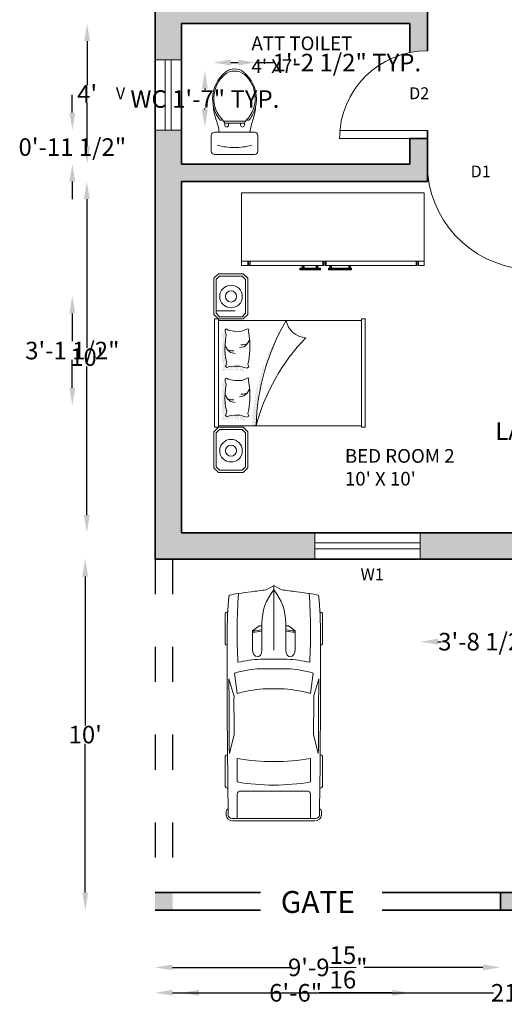
# Model space of a CAD drawing. Units: inches. Extents: x 2178 to 3409, y 1711 to 2279.
# Tile 1 of 8: x 2178 to 2343, y 1711 to 2047. Entities that reach past the tile are written whole.
import ezdxf

# ---------------------------------------------------------------- set-up
doc = ezdxf.new("R2010")
doc.units = ezdxf.units.IN
doc.linetypes.add('ACAD_ISO03W100', pattern=[30, 12, -18])
for name, color, linetype, lineweight in [('A-ANNO-DIMS', 2, 'Continuous', 18), ('A-ANNO-IDEN', 3, 'Continuous', 18), ('A-ANNO-TEXT', 7, 'Continuous', 18), ('A-AREA-IDEN', 7, 'Continuous', 18), ('A-DOOR', 4, 'Continuous', 18), ('A-EQPM-VEHI', 8, 'Continuous', 13), ('A-FURN', 8, 'Continuous', 18), ('A-GLAZ', 4, 'Continuous', 18), ('A-WALL', 7, 'Continuous', 35), ('A-WALL-HIDN', 7, 'ACAD_ISO03W100', 25), ('A-WALL-PATT', 252, 'Continuous', 13), ('WC-Detail_dwgmodels.com', 240, 'Continuous', 13), ('WC-Outline_dwgmodels.com', 250, 'Continuous', 18)]:
    doc.layers.add(name, color=color, linetype=linetype, lineweight=lineweight)
doc.styles.get("Standard").update_dxf_attribs({"font": 'arial.ttf'})
doc.dimstyles.get("Standard").update_dxf_attribs({"dimtxt": 6, "dimasz": 6, "dimexe": 0.18, "dimexo": 0.0625, "dimgap": 0.09, "dimtad": 0, "dimtih": 1, "dimtoh": 1, "dimdec": 4, "dimzin": 0, "dimdsep": 46, "dimlunit": 4, "dimtxsty": 'Standard', "dimcen": 0.09, "dimse1": 1, "dimse2": 1, "dimadec": 0, "dimazin": 0, "dimtfac": 1, "dimtdec": 4, "dimtofl": 0, "dimtmove": 0, "dimatfit": 3, "dimfxl": 1, "dimtolj": 1, "dimtzin": 0, "dimarcsym": 0})
pattern_1 = [(90, (3285.2007, -5256.0159), (-0.408110856, 0.204055428), [0, -0.408110856])]
pattern_2 = [(2e-12, (221.4576, -2145.7372), (1.73228346, -0.78740157), [11.8110236, -1.574803, 3.937008, -0.7874016]), (2e-12, (222.5049, -2146.1309), (-0.7874016, -1.0472441), [2.3622047, -0.2598425, 4.7244094, -0.5905512]), (2e-12, (221.8513, -2146.4065), (4.09448819, -0.52755906), [6.2992126, -1.1023622, 3.1496063, -0.7874016])]

# ---------------------------------------------------------------- blocks, each defined once
blk = doc.blocks.new('*U10')
for p, q in [((536, 950), (536, 936)), ((1182, 988), (568, 988)), ((1214, 950), (1214, 950)), ((2235, 810), (1899, 912)), ((3412, 904), (3030, 807)), ((3440, 942), (3440, 950)), ((3472, 988), (4087, 988)), ((4119, 950), (4119, 934)), ((4736, -851), (4736, 851)), ((4785, -832), (4785, 832)), ((1779, 801), (2195, 746)), ((3516, 746), (3994, 746)), ((4179, 670), (4179, -670)), ((4736, 746), (4242, 746)), ((820, 295), (918, 436)), ((918, 436), (1294, 436)), ((756, 241), (1313, 241)), ((816, 241), (816, 283)), ((1496, -274), (1496, 274)), ((1690, -267), (1690, 267)), ((2102, 216), (2102, -216)), ((4736, -267), (4736, 267)), ((83, 156), (3, 10)), ((0, 0), (1313, 0)), ((3, -10), (83, -156)), ((756, -241), (1313, -241)), ((816, -241), (816, -283)), ((820, -295), (918, -436)), ((918, -436), (1294, -436)), ((2195, -746), (1779, -801)), ((3994, -746), (3516, -746)), ((4242, -746), (4736, -746)), ((536, -950), (536, -936)), ((1182, -988), (568, -988)), ((1214, -950), (1214, -950)), ((2235, -810), (1899, -912)), ((3412, -904), (3030, -807)), ((3440, -942), (3440, -950)), ((3472, -988), (4087, -988)), ((4119, -950), (4119, -934))]:
    blk.add_line(p, q)
for centre, major_axis, ratio, start_param, end_param in [((6757, -699), (0, 7958), 0.842304, 1.367076, 1.39176), ((1046, -12468), (0, 13417), 0.842304, 0.00281, 0.075598), ((568, 950), (0, -37.6), 0.842304, 3.141593, 4.712389), ((1638, -268113), (0, 269063), 0.842304, -0.013397, 0.002797), ((1182, 950), (0, 37.6), 0.842304, -1.570796, 0), ((1638, -268113), (0, -269025), 0.842304, 3.133765, 3.140441), ((2433, -93125), (0, -93935), 0.842304, 3.134049, 3.144098), ((3472, 950), (0, -37.6), 0.842304, 3.141593, 4.712389), ((4087, 950), (0, 37.6), 0.842304, -1.570796, 0), ((4588, 910), (0, 56.4), 0.842304, -0.013017, 1.249894), ((1638, -268131), (0, 269121), 0.842304, -0.013397, -0.013017), ((4673, 851), (0, -75.2), 0.842304, 1.570796, 3.128196), ((4673, 832), (0, -133), 0.842304, 1.570796, 3.128196), ((6583, -699), (0, -7755), 0.842304, 4.528606, 4.561838), ((952, -15087), (0, -15833), 0.842304, 3.096046, 3.200911), ((3414, 137), (0, -2280), 0.842304, 4.449482, 4.652344), ((3436, 137), (0, 2077), 0.842304, 1.245306, 1.50788), ((3800, 71), (0, -2021), 0.842304, 4.372215, 4.640744), ((434, 0), (0, 3734), 0.842304, 4.511394, 4.913384), ((912, 0), (0, 3734), 0.842304, 4.511394, 4.913384), ((4242, 670), (0, 75.2), 0.842304, 0, 1.570796), ((-5194, 1331), (0, -6374), 0.842304, 1.385369, 1.434372), ((331, 432), (0, 696), 0.842304, 4.435146, 4.718221), ((361, 432), (0, 696), 0.842304, 4.435146, 4.718221), ((1290, 339), (161, -9), 0.603834, -1.395552, 1.581315), ((756, -1185), (0, 1427), 0.842304, 0, 0.590319), ((832, 283), (0, 18.8), 0.842304, 0.879714, 1.570796), ((16, 0), (0, -18.8), 0.842304, 4.131459, 5.293319), ((-5194, -1331), (0, 6374), 0.842304, -1.434372, -1.385369), ((756, 1185), (0, 1427), 0.842304, 2.551274, 3.141593), ((832, -283), (0, -18.8), 0.842304, 4.712389, 5.403472), ((331, -432), (0, -696), 0.842304, 1.564964, 1.848039), ((361, -432), (0, -696), 0.842304, 1.564964, 1.848039), ((3414, -137), (0, -2280), 0.842304, -1.510751, -1.307889), ((3436, -137), (0, -2077), 0.842304, -1.50788, -1.245306), ((3800, -71), (0, -2021), 0.842304, -1.499151, -1.230623), ((6583, 699), (0, 7755), 0.842304, 1.721348, 1.754579), ((6757, 699), (0, 7958), 0.842304, 1.749832, 1.774517), ((952, 15087), (0, -15833), 0.842304, -0.059319, 0.045547), ((4242, -670), (0, -75.2), 0.842304, 4.712389, 6.283185), ((1046, 12468), (0, -13417), 0.842304, -0.075598, -0.00281), ((568, -950), (0, 37.6), 0.842304, 1.570796, 3.141593), ((1638, 268113), (0, 269063), 0.842304, 3.138796, 3.15499), ((1182, -950), (0, -37.6), 0.842304, 0, 1.570796), ((1638, 268113), (0, -269025), 0.842304, 0.001152, 0.007828), ((2433, 93125), (0, -93935), 0.842304, -0.002505, 0.007544), ((3472, -950), (0, -37.6), 0.842304, -1.570796, 0), ((4087, -950), (0, 37.6), 0.842304, 3.141593, 4.712389), ((4588, -910), (0, -56.4), 0.842304, -1.249894, 0.013017), ((1638, 268131), (0, 269121), 0.842304, 3.15461, 3.15499), ((4673, -851), (0, 75.2), 0.842304, 3.15499, 4.712389), ((4673, -832), (0, -133), 0.842304, 0.013397, 1.570796)]:
    blk.add_ellipse(centre, major_axis=major_axis, ratio=ratio, start_param=start_param, end_param=end_param)
at = {"extrusion": (0, 0, -1)}
blk.add_ellipse((1290, -339), major_axis=(161, 9), ratio=0.603834, start_param=-1.395552, end_param=1.581315, dxfattribs=at)
blk = doc.blocks.new('*D13')
at = {"layer": 'A-ANNO-DIMS', "color": 0, "lineweight": -2, "transparency": 16777216}
for p, q in [((2200.86, 2040.04), (2200.86, 2025.13)), ((2200.86, 2004.04), (2200.86, 2018.95))]:
    blk.add_line(p, q, dxfattribs=at)
at = {"layer": 'A-ANNO-DIMS', "color": 0, "transparency": 16777216}
for points in [[(2199.86, 2040.04), (2201.86, 2040.04), (2200.86, 2046.04)], [(2199.86, 2004.04), (2201.86, 2004.04), (2200.86, 1998.04)]]:
    blk.add_solid(points, dxfattribs=at)
at = {"layer": 'Defpoints', "color": 0, "transparency": 16777216}
for p in [(2278.29, 2046.04), (2200.86, 1998.04), (2281.09, 1998.04)]:
    blk.add_point(p, dxfattribs=at)
at = {"layer": 'A-ANNO-DIMS', "color": 0, "transparency": 16777216, "insert": (2200.86, 2022.04), "char_height": 6, "width": 5.7626, "attachment_point": 5}
blk.add_mtext("\\A1;4'", dxfattribs=at)
blk = doc.blocks.new('*D14')
at = {"layer": 'A-ANNO-DIMS', "color": 0, "lineweight": -2, "transparency": 16777216}
for p, q in [((2200.76, 1986.04), (2200.76, 1935.2)), ((2200.76, 1878.04), (2200.76, 1928.89))]:
    blk.add_line(p, q, dxfattribs=at)
at = {"layer": 'A-ANNO-DIMS', "color": 0, "transparency": 16777216}
for points in [[(2199.76, 1986.04), (2201.76, 1986.04), (2200.76, 1992.04)], [(2199.76, 1878.04), (2201.76, 1878.04), (2200.76, 1872.04)]]:
    blk.add_solid(points, dxfattribs=at)
at = {"layer": 'Defpoints', "color": 0, "transparency": 16777216}
for p in [(2275.06, 1992.04), (2200.76, 1872.04), (2275.06, 1872.04)]:
    blk.add_point(p, dxfattribs=at)
at = {"layer": 'A-ANNO-DIMS', "color": 0, "transparency": 16777216, "insert": (2200.76, 1932.04), "char_height": 6, "attachment_point": 5}
blk.add_mtext("\\A1;10'", dxfattribs=at)
blk = doc.blocks.new('*D15')
at = {"layer": 'A-ANNO-DIMS', "color": 0, "lineweight": -2, "transparency": 16777216}
for p, q in [((2200.22, 1857.04), (2200.22, 1806.2)), ((2200.22, 1749.04), (2200.22, 1799.89))]:
    blk.add_line(p, q, dxfattribs=at)
at = {"layer": 'A-ANNO-DIMS', "color": 0, "transparency": 16777216}
for points in [[(2199.22, 1857.04), (2201.22, 1857.04), (2200.22, 1863.04)], [(2199.22, 1749.04), (2201.22, 1749.04), (2200.22, 1743.04)]]:
    blk.add_solid(points, dxfattribs=at)
at = {"layer": 'Defpoints', "color": 0, "transparency": 16777216}
for p in [(2238.48, 1863.04), (2200.22, 1743.04), (2238.48, 1743.04)]:
    blk.add_point(p, dxfattribs=at)
at = {"layer": 'A-ANNO-DIMS', "color": 0, "transparency": 16777216, "insert": (2200.22, 1803.04), "char_height": 6, "attachment_point": 5}
blk.add_mtext("\\A1;10'", dxfattribs=at)
blk = doc.blocks.new('*D16')
at = {"layer": 'A-ANNO-DIMS', "color": 0, "lineweight": -2, "transparency": 16777216}
for p, q in [((2230.06, 1723.48), (2270.74, 1723.48)), ((2336.02, 1723.48), (2295.35, 1723.48))]:
    blk.add_line(p, q, dxfattribs=at)
at = {"layer": 'A-ANNO-DIMS', "color": 0, "transparency": 16777216}
for points in [[(2230.06, 1724.48), (2230.06, 1722.48), (2224.06, 1723.48)], [(2336.02, 1724.48), (2336.02, 1722.48), (2342.02, 1723.48)]]:
    blk.add_solid(points, dxfattribs=at)
at = {"layer": 'Defpoints', "color": 0, "transparency": 16777216}
for p in [(2224.06, 1743.04), (2342.02, 1743.04), (2342.02, 1723.48)]:
    blk.add_point(p, dxfattribs=at)
at = {"layer": 'A-ANNO-DIMS', "color": 0, "transparency": 16777216, "insert": (2283.04, 1723.48), "char_height": 6, "attachment_point": 5}
blk.add_mtext('\\A1;9\'-9{\\H1x;\\S15/16;}"', dxfattribs=at)
blk = doc.blocks.new('BED-WITH-NIGHTSTANDS')
h = blk.add_hatch()
h.set_pattern_fill('DOTS', color=256, scale=0.257078, angle=90, style=0)
h.set_pattern_definition(pattern_1)
h.paths.add_polyline_path([(12.63, 18.62), (14.4, 18.62, -0.124273), (24.68, 54.62, 0.122563)])
h = blk.add_hatch()
h.set_pattern_fill('DOTS', color=256, scale=0.257078, angle=90, style=0)
h.set_pattern_definition(pattern_1)
h.paths.add_polyline_path([(3.05, 33.63), (2.57, 33.32), (2.57, 32.61), (2.97, 31.58), (2.65, 29.84), (2.42, 26.52), (2.65, 23.75), (3.13, 22.32), (2.65, 20.82), (3.28, 20.43), (4, 20.74), (5.81, 20.9), (7.55, 20.9), (9.13, 20.51), (10, 20.27), (10.71, 20.66), (10.32, 21.53), (10.39, 21.79), (8.83, 22.19), (7.1, 22.19), (5.28, 22.03), (4.57, 21.71), (3.93, 22.11), (4.41, 23.61), (3.93, 25.03), (3.7, 27.8), (3.93, 31.12), (4.25, 32.86), (4.14, 33.14), (3.6, 33.24)])
h.paths.add_polyline_path([(3.05, 50.43), (2.57, 50.11), (2.57, 49.4), (2.97, 48.37), (2.65, 46.63), (2.42, 43.31), (2.65, 40.54), (3.13, 39.12), (2.65, 37.62), (3.28, 37.22), (4, 37.54), (5.81, 37.7), (7.55, 37.7), (9.13, 37.3), (10, 37.06), (10.71, 37.46), (10.32, 38.33), (10.39, 38.59), (8.83, 38.98), (7.1, 38.98), (5.28, 38.82), (4.57, 38.51), (3.93, 38.9), (4.41, 40.4), (3.93, 41.83), (3.7, 44.59), (3.93, 47.92), (4.25, 49.66), (4.14, 49.93), (3.6, 50.03)])
for p, q in [((0.8, 57.9), (7.23, 57.9)), ((0.26, 55.13), (0.26, 18.11)), ((0.26, 55.13), (1.54, 55.13)), ((1.54, 55.13), (1.54, 18.11)), ((1.54, 54.62), (50.39, 54.62)), ((50.39, 55.13), (50.39, 18.11)), ((50.39, 55.13), (51.67, 55.13)), ((51.67, 55.13), (51.67, 18.11)), ((1.54, 18.11), (0.26, 18.11)), ((50.39, 18.62), (1.54, 18.62)), ((51.67, 18.11), (50.39, 18.11))]:
    blk.add_line(p, q)
for points in [[(11.57, 56.67), (11.57, 69.01), (10.03, 70.55), (1.54, 70.55), (0, 69.01), (0, 56.67), (1.54, 55.13), (10.03, 55.13)], [(10.8, 57.06), (10.8, 68.63), (9.64, 69.78), (1.93, 69.78), (0.77, 68.63), (0.77, 57.06), (1.93, 55.9), (9.64, 55.9)], [(11.57, 4.23), (11.57, 16.57), (10.03, 18.11), (1.54, 18.11), (0, 16.57), (0, 4.23), (1.54, 2.69), (10.03, 2.69)], [(10.8, 4.61), (10.8, 16.18), (9.64, 17.34), (1.93, 17.34), (0.77, 16.18), (0.77, 4.61), (1.93, 3.46), (9.64, 3.46)]]:
    blk.add_lwpolyline(points, close=True)
for points in [[(4.41, 40.4), (3.93, 38.9), (4.57, 38.51), (5.28, 38.82), (7.1, 38.98), (8.83, 38.98), (10.41, 38.58), (11.28, 38.35), (11.99, 38.74), (11.6, 39.61), (11.99, 40.96), (12.23, 44.2), (12.23, 47.52), (11.84, 51), (11.99, 51.63), (11.6, 51.79), (10.97, 51.47), (9.54, 50.92), (7.17, 50.84), (5.75, 51.16), (4.88, 51.32), (4.33, 51.71), (3.86, 51.4), (3.86, 50.68), (4.25, 49.66), (3.93, 47.92), (3.7, 44.59), (3.93, 41.83), (4.41, 40.4)], [(12.15, 47.92), (11.36, 46.57), (10.33, 45.62), (8.75, 45.31)], [(3.86, 45.94), (4.65, 44.59), (5.67, 43.65), (7.25, 43.33)], [(4.72, 44.59), (5.99, 44.28), (6.78, 44.28)], [(11.28, 46.57), (10.02, 46.26), (9.23, 46.26)], [(4.41, 23.61), (3.93, 22.11), (4.57, 21.71), (5.28, 22.03), (7.1, 22.19), (8.83, 22.19), (10.41, 21.79), (11.28, 21.55), (11.99, 21.95), (11.6, 22.82), (11.99, 24.16), (12.23, 27.4), (12.23, 30.73), (11.84, 34.21), (11.99, 34.84), (11.6, 35), (10.97, 34.68), (9.54, 34.13), (7.17, 34.05), (5.75, 34.36), (4.88, 34.52), (4.33, 34.92), (3.86, 34.6), (3.86, 33.89), (4.25, 32.86), (3.93, 31.12), (3.7, 27.8), (3.93, 25.03), (4.41, 23.61)], [(12.15, 31.12), (11.36, 29.78), (10.33, 28.83), (8.75, 28.51)], [(3.86, 29.14), (4.65, 27.8), (5.67, 26.85), (7.25, 26.53)], [(4.72, 27.8), (5.99, 27.48), (6.78, 27.48)], [(11.28, 29.78), (10.02, 29.46), (9.23, 29.46)]]:
    blk.add_lwpolyline(points)
for centre, radius in [((5.86, 62.82), 3.86), ((5.86, 62.82), 1.91), ((5.86, 10.09), 3.86), ((5.86, 10.09), 1.91)]:
    blk.add_circle(centre, radius)
for centre, radius, start, end in [((90.82, 16.25), 76.46, 149.8866, 178.2226), ((31.77, 55.91), 7.21, 190.3543, 266.7862), ((82.59, 0), 70.69, 136.4367, 164.7234)]:
    blk.add_arc(centre, radius, start, end)
blk = doc.blocks.new('BEDROOM-WARDROBE')
h = blk.add_hatch()
h.set_pattern_fill('AR-RROOF', color=256, scale=0.787402, angle=360, style=0)
h.set_pattern_definition(pattern_2)
h.paths.add_polyline_path([(19.88, 0.59), (19.88, 0), (26.97, 0), (26.97, 0.59)])
h.paths.add_polyline_path([(26.07, 1.57), (25.48, 1.57), (25.48, 0.59), (26.07, 0.59)])
h.paths.add_polyline_path([(21.37, 1.57), (20.78, 1.57), (20.78, 0.59), (21.37, 0.59)])
h = blk.add_hatch()
h.set_pattern_fill('AR-RROOF', color=256, scale=0.787402, angle=360, style=0)
h.set_pattern_definition(pattern_2)
h.paths.add_polyline_path([(29.73, 0.59), (29.73, 0), (37.6, 0), (37.6, 0.59)])
h.paths.add_polyline_path([(37.21, 1.57), (36.61, 1.57), (36.61, 0.59), (37.21, 0.59)])
h.paths.add_polyline_path([(30.71, 0.59), (30.71, 1.57), (30.12, 1.57), (30.12, 0.59)])
for p, q in [((0, 26.38), (62.4, 26.38)), ((0, 26.38), (0, 1.57)), ((62.4, 26.38), (62.4, 1.74)), ((62.4, 2.95), (0, 2.95)), ((0, 1.57), (2.17, 1.57)), ((2.17, 1.57), (2.17, 2.95)), ((2.56, 1.54), (2.56, 2.95)), ((2.95, 1.54), (2.56, 1.54)), ((2.95, 1.57), (2.95, 2.95)), ((27.76, 1.57), (2.95, 1.57)), ((2.95, 1.57), (2.95, 1.54)), ((19.88, 0.59), (26.97, 0.59)), ((19.88, 0), (19.88, 0.59)), ((26.97, 0), (19.88, 0)), ((20.78, 0.59), (20.78, 1.57)), ((21.37, 0.59), (21.37, 1.57)), ((25.48, 0.59), (25.48, 1.57)), ((26.07, 0.59), (26.07, 1.57)), ((26.97, 0.59), (26.97, 0)), ((27.76, 2.95), (27.76, 1.57)), ((27.76, 1.54), (27.76, 1.57)), ((28.15, 1.54), (27.76, 1.54)), ((28.15, 2.95), (28.15, 1.54)), ((28.54, 2.95), (28.54, 1.54)), ((28.54, 1.54), (28.94, 1.54)), ((28.94, 2.95), (28.94, 1.57)), ((28.94, 1.57), (59.65, 1.57)), ((28.94, 1.54), (28.94, 1.57)), ((29.73, 0.59), (37.6, 0.59)), ((29.73, 0), (29.73, 0.59)), ((37.6, 0), (29.73, 0)), ((30.12, 0.59), (30.12, 1.57)), ((30.71, 0.59), (30.71, 1.57)), ((36.61, 0.59), (36.61, 1.57)), ((37.21, 0.59), (37.21, 1.57)), ((37.6, 0.59), (37.6, 0)), ((59.65, 2.95), (59.65, 1.57)), ((59.65, 1.57), (59.65, 1.54)), ((59.65, 1.54), (60.04, 1.54)), ((60.04, 1.54), (60.04, 2.95)), ((60.43, 2.95), (60.43, 1.57))]:
    blk.add_line(p, q)
for centre, radius, start, end in [((61.42, 6.59), 5.11, 258.8892, 279.227), ((62.2, 1.74), 0.197, 279.227, 0)]:
    blk.add_arc(centre, radius, start, end)
blk = doc.blocks.new('WC-SEAT-ASSEMBLY')
for p, q in [((3.53, 1.38), (3.89, 0.72)), ((5.18, 0.72), (3.89, 0.72)), ((3.89, 0.72), (3.89, 0)), ((7.25, 0.72), (5.18, 0.72)), ((5.18, 0), (5.18, 0.72)), ((7.25, 0.72), (9.32, 0.72)), ((9.32, 0.72), (10.61, 0.72)), ((9.32, 0), (9.32, 0.72)), ((10.97, 1.38), (10.61, 0.72)), ((10.61, 0.72), (10.61, 0))]:
    blk.add_line(p, q)
for points in [[(3.26, 1.65, -0.434217), (3.89, 17.29, -0.182634), (7.25, 18.51, -2.693815)], [(11.24, 1.65, 0.434217), (10.61, 17.29, 0.182634), (7.25, 18.51, 2.693815)], [(0.16, 6.03, -0.015301), (0, 6.73, -0.16845)], [(2.36, 1.65, -0.105447), (0.16, 6.03, -0.16845)], [(12.14, 1.65, 0.094048), (14.19, 5.52, 0.16845)], [(14.19, 5.52, 0.026594), (14.5, 6.73, 0.16845)], [(3.26, 1.65), (2.36, 1.65, -0.416606)], [(3.53, 1.38, -0.008985), (3.26, 1.65, -0.182634)], [(7.25, 1.38), (3.53, 1.38, -0.444938)], [(7.25, 1.38), (10.97, 1.38, 0.008985)], [(10.97, 1.38, 0.008985), (11.24, 1.65, 0.182634)], [(11.24, 1.65), (12.14, 1.65, 0.416606)]]:
    blk.add_lwpolyline(points, format="xyb")
for centre in [(4.54, 0), (9.96, 0)]:
    blk.add_arc(centre, 0.645, 180, 0)
blk = doc.blocks.new('WINDOW-36')
for p, q in [((36, 9), (0, 9)), ((0, 9), (0, 0)), ((36, 0), (36, 9)), ((0, 5.5), (36, 5.5)), ((0, 3.5), (36, 3.5)), ((0, 0), (36, 0))]:
    blk.add_line(p, q)
blk = doc.blocks.new('VENT-24')
for p, q in [((9, 24), (0, 24)), ((0, 24), (0, 0)), ((3.5, 0), (3.5, 24)), ((5.5, 0), (5.5, 24)), ((9, 0), (9, 24)), ((0, 0), (9, 0))]:
    blk.add_line(p, q)
blk = doc.blocks.new('DOOR-30')
for p, q in [((-30, 2.75), (0, 2.75)), ((-30, 0), (0, 0)), ((0, 2.75), (0, 0))]:
    blk.add_line(p, q)
blk.add_arc((0, 0), 30, 90, 180)
blk = doc.blocks.new('DOOR-36')
for p, q in [((0, 0), (0, 36)), ((3, 0), (3, 35.87)), ((3, 0), (0, 0))]:
    blk.add_line(p, q)
blk.add_arc((0, 0), 36, 0, 85.2198)
blk = doc.blocks.new('*D45')
at = {"layer": 'A-ANNO-DIMS', "color": 0, "lineweight": -2, "transparency": 16777216}
for p, q in [((2377.15, 1916.05), (2377.15, 1922.05)), ((2377.15, 1897.4), (2377.15, 1891.4))]:
    blk.add_line(p, q, dxfattribs=at)
at = {"layer": 'A-ANNO-DIMS', "color": 0, "transparency": 16777216}
for points in [[(2376.15, 1916.05), (2378.15, 1916.05), (2377.15, 1910.05)], [(2376.15, 1897.4), (2378.15, 1897.4), (2377.15, 1903.4)]]:
    blk.add_solid(points, dxfattribs=at)
at = {"layer": 'Defpoints', "color": 0, "transparency": 16777216}
for p in [(2376.15, 1910.05), (2377.15, 1910.05), (2376.15, 1903.4)]:
    blk.add_point(p, dxfattribs=at)
at = {"layer": 'A-ANNO-DIMS', "color": 0, "transparency": 16777216, "insert": (2377.15, 1906.72), "char_height": 6, "attachment_point": 5}
blk.add_mtext('\\A1;LAMP 0\'-6 1/2" TYP.', dxfattribs=at)
blk = doc.blocks.new('*D51')
at = {"layer": 'A-ANNO-DIMS', "color": 0, "lineweight": -2, "transparency": 16777216}
for p, q in [((2241.08, 2023.86), (2241.08, 2023.46)), ((2241.08, 2016.69), (2241.08, 2017.08))]:
    blk.add_line(p, q, dxfattribs=at)
at = {"layer": 'A-ANNO-DIMS', "color": 0, "transparency": 16777216}
for points in [[(2240.08, 2023.86), (2242.08, 2023.86), (2241.08, 2029.86)], [(2240.08, 2016.69), (2242.08, 2016.69), (2241.08, 2010.69)]]:
    blk.add_solid(points, dxfattribs=at)
at = {"layer": 'Defpoints', "color": 0, "transparency": 16777216}
for p in [(2241.08, 2029.86), (2243.96, 2029.86), (2243.96, 2010.69)]:
    blk.add_point(p, dxfattribs=at)
at = {"layer": 'A-ANNO-DIMS', "color": 0, "transparency": 16777216, "insert": (2241.08, 2020.27), "char_height": 6, "attachment_point": 5}
blk.add_mtext('\\A1;WC 1\'-7" TYP.', dxfattribs=at)
blk = doc.blocks.new('*D52')
at = {"layer": 'A-ANNO-DIMS', "color": 0, "lineweight": -2, "transparency": 16777216}
for p, q in [((2249.96, 2032.73), (2252.46, 2032.73)), ((2258.46, 2032.73), (2264.46, 2032.73))]:
    blk.add_line(p, q, dxfattribs=at)
at = {"layer": 'A-ANNO-DIMS', "color": 0, "transparency": 16777216}
for points in [[(2249.96, 2033.73), (2249.96, 2031.73), (2243.96, 2032.73)], [(2252.46, 2033.73), (2252.46, 2031.73), (2258.46, 2032.73)]]:
    blk.add_solid(points, dxfattribs=at)
at = {"layer": 'Defpoints', "color": 0, "transparency": 16777216}
for p in [(2258.46, 2032.73), (2243.96, 2029.86), (2258.46, 2029.86)]:
    blk.add_point(p, dxfattribs=at)
at = {"layer": 'A-ANNO-DIMS', "color": 0, "transparency": 16777216, "insert": (2289.54, 2032.73), "char_height": 6, "attachment_point": 5}
blk.add_mtext('\\A1;1\'-2 1/2" TYP.', dxfattribs=at)
blk = doc.blocks.new('*D53')
at = {"layer": 'A-ANNO-DIMS', "color": 0, "lineweight": -2, "transparency": 16777216}
for p, q in [((2293.06, 2057.04), (2311.06, 2057.04)), ((2317.06, 2057.04), (2323.06, 2057.04))]:
    blk.add_line(p, q, dxfattribs=at)
at = {"layer": 'A-ANNO-DIMS', "color": 0, "transparency": 16777216}
for points in [[(2293.06, 2058.04), (2293.06, 2056.04), (2287.06, 2057.04)], [(2311.06, 2058.04), (2311.06, 2056.04), (2317.06, 2057.04)]]:
    blk.add_solid(points, dxfattribs=at)
at = {"layer": 'Defpoints', "color": 0, "transparency": 16777216}
for p in [(2287.06, 2061.54), (2317.06, 2061.54), (2317.06, 2057.04)]:
    blk.add_point(p, dxfattribs=at)
at = {"layer": 'A-ANNO-DIMS', "color": 0, "transparency": 16777216, "insert": (2347.81, 2057.04), "char_height": 6, "attachment_point": 5}
blk.add_mtext('\\A1;D2 2\'-6" TYP.', dxfattribs=at)
blk = doc.blocks.new('*D61')
at = {"layer": 'A-ANNO-DIMS', "color": 0, "lineweight": -2, "transparency": 16777216}
for p, q in [((2239.06, 1714.79), (2263.98, 1714.79)), ((2305.06, 1714.79), (2280.15, 1714.79))]:
    blk.add_line(p, q, dxfattribs=at)
at = {"layer": 'A-ANNO-DIMS', "color": 0, "transparency": 16777216}
for points in [[(2239.06, 1715.79), (2239.06, 1713.79), (2233.06, 1714.79)], [(2305.06, 1715.79), (2305.06, 1713.79), (2311.06, 1714.79)]]:
    blk.add_solid(points, dxfattribs=at)
at = {"layer": 'Defpoints', "color": 0, "transparency": 16777216}
for p in [(2233.06, 1998.04), (2311.06, 1998.04), (2311.06, 1714.79)]:
    blk.add_point(p, dxfattribs=at)
at = {"layer": 'A-ANNO-DIMS', "color": 0, "transparency": 16777216, "insert": (2272.06, 1714.79), "char_height": 6, "attachment_point": 5}
blk.add_mtext('\\A1;6\'-6"', dxfattribs=at)
blk = doc.blocks.new('*D63')
at = {"layer": 'A-ANNO-DIMS', "color": 0, "lineweight": -2, "transparency": 16777216}
for p, q in [((2195.814847, 2015.642505), (2195.814847, 2021.642505)), ((2195.814847, 1992.042563), (2195.814847, 1986.042563))]:
    blk.add_line(p, q, dxfattribs=at)
at = {"layer": 'A-ANNO-DIMS', "color": 0, "transparency": 16777216}
for points in [[(2194.814847, 2015.642505), (2196.814847, 2015.642505), (2195.814847, 2009.642505)], [(2194.814847, 1992.042563), (2196.814847, 1992.042563), (2195.814847, 1998.042563)]]:
    blk.add_solid(points, dxfattribs=at)
at = {"layer": 'Defpoints', "color": 0, "transparency": 16777216}
for p in [(2195.814847, 2009.642505), (2233.064847, 2009.642505), (2233.064847, 1998.042563)]:
    blk.add_point(p, dxfattribs=at)
at = {"layer": 'A-ANNO-DIMS', "color": 0, "transparency": 16777216, "insert": (2195.814847, 2003.842534), "char_height": 6, "attachment_point": 5}
blk.add_mtext('\\A1;0\'-11 1/2"', dxfattribs=at)
blk = doc.blocks.new('*D68')
at = {"layer": 'A-ANNO-DIMS', "color": 0, "lineweight": -2, "transparency": 16777216}
for p, q in [((2320.65, 1834.79), (2321.8, 1834.79)), ((2353.06, 1834.79), (2351.91, 1834.79))]:
    blk.add_line(p, q, dxfattribs=at)
at = {"layer": 'A-ANNO-DIMS', "color": 0, "transparency": 16777216}
for points in [[(2320.65, 1835.79), (2320.65, 1833.79), (2314.65, 1834.79)], [(2353.06, 1835.79), (2353.06, 1833.79), (2359.06, 1834.79)]]:
    blk.add_solid(points, dxfattribs=at)
at = {"layer": 'Defpoints', "color": 0, "transparency": 16777216}
for p in [(2314.65, 1863.04), (2359.06, 1863.04), (2314.65, 1834.79)]:
    blk.add_point(p, dxfattribs=at)
at = {"layer": 'A-ANNO-DIMS', "color": 0, "transparency": 16777216, "insert": (2336.86, 1834.79), "char_height": 6, "attachment_point": 5}
blk.add_mtext('\\A1;3\'-8 1/2"', dxfattribs=at)
blk = doc.blocks.new('*D72')
at = {"layer": 'A-ANNO-DIMS', "color": 0, "lineweight": -2, "transparency": 16777216}
for p, q in [((2195.81, 1946.99), (2195.81, 1937.48)), ((2195.81, 1921.59), (2195.81, 1931.1))]:
    blk.add_line(p, q, dxfattribs=at)
at = {"layer": 'A-ANNO-DIMS', "color": 0, "transparency": 16777216}
for points in [[(2194.81, 1946.99), (2196.81, 1946.99), (2195.81, 1952.99)], [(2194.81, 1921.59), (2196.81, 1921.59), (2195.81, 1915.59)]]:
    blk.add_solid(points, dxfattribs=at)
at = {"layer": 'Defpoints', "color": 0, "transparency": 16777216}
for p in [(2195.81, 1952.99), (2366.59, 1952.99), (2366.59, 1915.59)]:
    blk.add_point(p, dxfattribs=at)
at = {"layer": 'A-ANNO-DIMS', "color": 0, "transparency": 16777216, "insert": (2195.81, 1934.29), "char_height": 6, "attachment_point": 5}
blk.add_mtext('\\A1;3\'-1 1/2"', dxfattribs=at)
blk = doc.blocks.new('*D74')
at = {"layer": 'A-ANNO-DIMS', "color": 0, "lineweight": -2, "transparency": 16777216}
for p, q in [((2230.06, 1714.79), (2339.62, 1714.79)), ((2470.06, 1714.79), (2360.51, 1714.79))]:
    blk.add_line(p, q, dxfattribs=at)
at = {"layer": 'A-ANNO-DIMS', "color": 0, "transparency": 16777216}
for points in [[(2230.06, 1715.79), (2230.06, 1713.79), (2224.06, 1714.79)], [(2470.06, 1715.79), (2470.06, 1713.79), (2476.06, 1714.79)]]:
    blk.add_solid(points, dxfattribs=at)
at = {"layer": 'Defpoints', "color": 0, "transparency": 16777216}
for p in [(2224.06, 1743.04), (2476.06, 1743.04), (2476.06, 1714.79)]:
    blk.add_point(p, dxfattribs=at)
at = {"layer": 'A-ANNO-DIMS', "color": 0, "transparency": 16777216, "insert": (2350.06, 1714.79), "char_height": 6, "attachment_point": 5}
blk.add_mtext('\\A1;21\'-0"', dxfattribs=at)

msp = doc.modelspace()

# ---------------------------------------------------------------- hatches: boundary and pattern name
at = {"layer": 'A-WALL-PATT'}
h = msp.add_hatch(color=256, dxfattribs=at)
h.dxf.hatch_style = 1
h.paths.add_polyline_path([(2233.06485, 1992.04256), (2317.06485, 1992.04256), (2317.06485, 1998.04256), (2317.06485, 2006.75072), (2311.06485, 2006.75072), (2311.06485, 1998.04256), (2233.06485, 1998.04256), (2233.06485, 2009.64251), (2224.06485, 2009.64251), (2224.06485, 1863.04256), (2233.06485, 1863.04256), (2278.65041, 1863.04256), (2278.65041, 1872.04256), (2233.06485, 1872.04256)])
h.paths.add_polyline_path([(2359.06485, 1992.04256), (2359.06485, 1998.04256), (2353.06485, 1998.04256), (2353.06485, 1962.04256), (2353.06485, 1872.04256), (2314.65041, 1872.04256), (2314.65041, 1863.04256), (2359.06485, 1863.04256), (2359.06485, 1872.04256)])
h.paths.add_polyline_path([(2401.06485, 1890.04256), (2371.06485, 1890.04256), (2359.06485, 1890.04256), (2359.06485, 1884.04256), (2371.06485, 1884.04256), (2377.06485, 1884.04256), (2401.06485, 1884.04256)])
h.paths.add_polyline_path([(2353.06485, 1802.77269), (2359.06485, 1802.77269), (2359.06485, 1808.77269), (2356.83755, 1808.77269), (2353.06485, 1808.77269), (2347.91295, 1808.77269), (2347.91295, 1802.77269), (2347.91295, 1749.04256), (2342.02347, 1749.04256), (2342.02347, 1743.04256), (2353.06485, 1743.04256)])
h.paths.add_polyline_path([(2476.06485, 2247.04256), (2442.91353, 2247.04256), (2442.91353, 2238.04256), (2467.06485, 2238.04256), (2467.06485, 2041.93675), (2476.06485, 2041.93675)])
h.paths.add_polyline_path([(2467.06485, 2106.04256), (2406.56133, 2106.04256, -0.04188649), (2407.06485, 2100.04256), (2467.06485, 2100.04256)])
h.paths.add_polyline_path([(2406.91353, 2247.04256), (2321.22384, 2247.04256), (2321.22384, 2238.04256), (2365.06485, 2238.04256), (2365.06485, 2106.04256), (2365.06485, 2100.04256), (2371.06485, 2100.04256), (2371.06485, 2136.04256), (2371.06485, 2238.04256), (2406.91353, 2238.04256)])
h.paths.add_polyline_path([(2285.22384, 2247.04256), (2224.06485, 2247.04256), (2224.06485, 2087.1459), (2233.06485, 2087.1459), (2233.06485, 2100.04256), (2329.06485, 2100.04256, -0.04188649), (2329.56837, 2106.04256), (2233.06485, 2106.04256), (2233.06485, 2238.04256), (2285.22384, 2238.04256)])
h.paths.add_polyline_path([(2317.06485, 2052.04256), (2317.06485, 2061.5418), (2311.06485, 2061.5418), (2311.06485, 2052.04256), (2233.06485, 2052.04256), (2233.06485, 2063.1459), (2224.06485, 2063.1459), (2224.06485, 2033.64251), (2233.06485, 2033.64251), (2233.06485, 2046.04256), (2311.06485, 2046.04256), (2311.06485, 2036.1446, -0.050382044), (2317.06485, 2036.75072), (2317.06485, 2046.04256)])
h = msp.add_hatch(color=256, dxfattribs=at)
h.dxf.hatch_style = 1
h.paths.add_polyline_path([(2230.06485, 1749.04256), (2224.06485, 1749.04256), (2224.06485, 1743.04256), (2230.06485, 1743.04256)])

# ---------------------------------------------------------------- linework, layer by layer
at = {"layer": 'A-WALL'}
for p, q in [((2224.06485, 2247.04256), (2224.06485, 1863.04256)), ((2317.06485, 2052.04256), (2317.06485, 2046.04256)), ((2233.06485, 2046.04256), (2311.06485, 2046.04256)), ((2233.06485, 2046.04256), (2233.06485, 1998.04256)), ((2311.06485, 2046.04256), (2311.06485, 2036.1446)), ((2317.06485, 2046.04256), (2317.06485, 2036.75072)), ((2317.06485, 2009.50072), (2317.06485, 1998.04256)), ((2311.06485, 2006.75072), (2317.06485, 2006.75072)), ((2311.06485, 2006.75072), (2311.06485, 1998.04256)), ((2233.06485, 1998.04256), (2311.06485, 1998.04256)), ((2317.06485, 1998.04256), (2317.06485, 1992.04256)), ((2233.06485, 1992.04256), (2317.06485, 1992.04256)), ((2233.06485, 1992.04256), (2233.06485, 1872.04256)), ((2317.06485, 1992.04256), (2317.06485, 1992.04256)), ((2233.06485, 1872.04256), (2353.06485, 1872.04256)), ((2233.06485, 1863.04256), (2224.06485, 1863.04256)), ((2233.06485, 1863.04256), (2359.06485, 1863.04256)), ((2224.06485, 1749.04256), (2260.12659, 1749.04256)), ((2301.6348, 1749.04256), (2347.91295, 1749.04256)), ((2342.02347, 1749.04256), (2342.02347, 1743.04256)), ((2224.06485, 1743.04256), (2260.12659, 1743.04256)), ((2301.6348, 1743.04256), (2353.06485, 1743.04256))]:
    msp.add_line(p, q, dxfattribs=at)
at = {"layer": 'A-WALL-HIDN'}
for p, q in [((2224.06485, 1863.04256), (2224.06485, 1743.04256)), ((2230.06485, 1863.04256), (2230.06485, 1743.04256))]:
    msp.add_line(p, q, dxfattribs=at)
at = {"layer": 'WC-Detail_dwgmodels.com'}
for centre, start, end in [((2251.2188, 2026.93984), 255.3287681, 269.9720383), ((2251.19609, 2026.93984), 270.0279617, 284.6712319)]:
    msp.add_arc(centre, 23.26046, start, end, dxfattribs=at)
at = {"layer": 'WC-Outline_dwgmodels.com'}
for points in [[(2243.73671, 2020.29899, -0.230343354), (2248.20821, 2029.54924, -0.168450027), (2251.20745, 2030.58986, -2.883081922)], [(2258.67818, 2020.29899, 0.230343354), (2254.20668, 2029.54924, 0.168450027), (2251.20745, 2030.58986, 2.883081922)], [(2243.958, 2018.05942, -0.048022765), (2243.73671, 2020.29899, -0.168450027)], [(2258.45689, 2018.05942, 0.048022765), (2258.67818, 2020.29899, 0.168450027)], [(2244.41702, 2008.91103, 0.414213562), (2243.27883, 2007.77284), (2243.27883, 2002.46745, 0.414213562), (2244.41702, 2001.32926), (2251.20745, 2001.32926), (2257.99787, 2001.32926, 0.414213562), (2259.13606, 2002.46745), (2259.13606, 2007.77284, 0.414213562), (2257.99787, 2008.91103), (2256.44246, 2008.91103, -0.052345057), (2257.46672, 2013.15682, 0.071131414), (2258.45689, 2018.05942, 0.160777477)], [(2243.958, 2018.05942, 0.071131414), (2244.94817, 2013.15682, -0.052345057), (2245.97243, 2008.91103), (2244.41702, 2008.91103, 0.414213562)], [(2245.97243, 2008.91103), (2251.20745, 2008.91103, -0.414213562)], [(2256.44246, 2008.91103), (2251.20745, 2008.91103, 0.414213562)]]:
    msp.add_lwpolyline(points, format="xyb", dxfattribs=at)

# ---------------------------------------------------------------- block references
at = {"layer": 'A-DOOR'}
msp.add_blockref('DOOR-30', (2317.06485, 2006.75072), dxfattribs=at)
at = {"layer": 'A-DOOR', "rotation": 180}
msp.add_blockref('DOOR-36', (2353.06485, 1998.04256), dxfattribs=at)
at = {"layer": 'A-EQPM-VEHI', "xscale": 0.0168018776673516, "yscale": 0.0168018776673516, "zscale": 0.0168018776673516, "rotation": 270}
msp.add_blockref('*U10', (2264.62777, 1853.94884), dxfattribs=at)
at = {"layer": 'A-FURN'}
for name, p in [('BEDROOM-WARDROBE', (2253.57147, 1961.84621)), ('BED-WITH-NIGHTSTANDS', (2244.14407, 1889.97743))]:
    msp.add_blockref(name, p, dxfattribs=at)
at = {"layer": 'A-GLAZ'}
for name, p in [('VENT-24', (2224.06485, 2009.64251)), ('WINDOW-36', (2278.65041, 1863.04256))]:
    msp.add_blockref(name, p, dxfattribs=at)
at = {"layer": 'WC-Detail_dwgmodels.com'}
msp.add_blockref('WC-SEAT-ASSEMBLY', (2243.958, 2011.3324), dxfattribs=at)

# ---------------------------------------------------------------- texts
at = {"layer": 'A-ANNO-IDEN', "attachment_point": 1}
for s, insert, char_height in [('V', (2210.68353, 2024.26513), 4.05121), ('D2', (2310.82239, 2024.26513), 4.051205), ('D1', (2331.82395, 1997.5435), 4.051205), ('W1', (2294.24715, 1859.83037), 4.051205)]:
    msp.add_mtext_dynamic_manual_height_columns(s, width=167.0263497, gutter_width=20.25603, heights=[0], dxfattribs=dict(at, insert=insert, char_height=char_height))
at = {"layer": 'A-ANNO-TEXT', "insert": (2266.99709, 1749.5702), "char_height": 7.470133, "attachment_point": 1}
msp.add_mtext_dynamic_manual_height_columns('GATE ', width=86.0282639, gutter_width=37.35066, heights=[0], dxfattribs=at)
at = {"layer": 'A-AREA-IDEN', "char_height": 4.679699, "attachment_point": 1}
for s, insert in [("ATT TOILET\\P4' X7'", (2256.97802, 2041.63997)), ("BED ROOM 2\\P10' X 10'", (2288.89227, 1900.62715))]:
    msp.add_mtext_dynamic_manual_height_columns(s, width=123.0595467, gutter_width=23.3985, heights=[41.64659], dxfattribs=dict(at, insert=insert))

# ---------------------------------------------------------------- dimensions: what is measured, and where the dimension line sits
at = {"layer": 'A-ANNO-DIMS'}
for base, p1, p2, text, picture, middle in [((2317.06485, 2057.0418), (2287.06485, 2061.5418), (2317.06485, 2061.5418), 'D2 <> TYP.', '*D53', (2347.81378, 2057.0418)), ((2258.45689, 2032.7325), (2243.958, 2029.85704), (2258.45689, 2029.85704), '<> TYP.', '*D52', (2289.54144, 2032.7325))]:
    dim = msp.add_linear_dim(base=base, p1=p1, p2=p2, text=text, dimstyle='Standard', override={"dimdec": 1, "dimlfac": 1, "dimrnd": 0, "dimzin": 1, "dimdsep": 46, "dimlunit": 4, "dimfrac": 2}, dxfattribs=at)
    dim.commit()
    dim.dimension.update_dxf_attribs({"geometry": picture, "text_midpoint": middle})
for base, p1, p2, angle, override, picture, middle in [((2200.86415, 1998.04256), (2278.28695, 2046.04256), (2281.08959, 1998.04256), 90, {"dimclrd": 0, "dimclre": 0, "dimclrt": 0}, '*D13', (2200.86415, 2022.04256)), ((2195.81485, 2009.64251), (2233.06485, 1998.04256), (2233.06485, 2009.64251), 90, {"dimdec": 1, "dimlfac": 1, "dimrnd": 0, "dimzin": 1, "dimdsep": 46, "dimlunit": 4, "dimfrac": 2}, '*D63', (2195.81485, 2003.84253)), ((2200.76042, 1872.04256), (2275.06485, 1992.04256), (2275.06485, 1872.04256), 90, {"dimclrd": 0, "dimclre": 0, "dimclrt": 0}, '*D14', (2200.76042, 1932.04256)), ((2195.81485, 1952.986), (2366.59328, 1915.59289), (2366.59328, 1952.986), 90, {"dimdec": 1, "dimlfac": 1, "dimrnd": 0, "dimzin": 1, "dimdsep": 46, "dimlunit": 4, "dimfrac": 2}, '*D72', (2195.81485, 1934.28944)), ((2200.22424, 1743.04256), (2238.47725, 1863.04256), (2238.47725, 1743.04256), 90, {"dimclrd": 0, "dimclre": 0, "dimclrt": 0}, '*D15', (2200.22424, 1803.04256)), ((2314.65041, 1834.79256), (2359.06485, 1863.04256), (2314.65041, 1863.04256), 180, {"dimdec": 1, "dimlfac": 1, "dimrnd": 0, "dimzin": 1, "dimdsep": 46, "dimlunit": 4, "dimfrac": 2}, '*D68', (2336.85763, 1834.79256))]:
    dim = msp.add_linear_dim(base=base, p1=p1, p2=p2, angle=angle, dimstyle='Standard', override=override, dxfattribs=at)
    dim.commit()
    dim.dimension.update_dxf_attribs({"geometry": picture, "text_midpoint": middle})
for base, p1, p2, text, picture, middle in [((2241.08253, 2029.85704), (2243.958, 2010.68728), (2243.958, 2029.85704), 'WC <> TYP.', '*D51', (2241.08253, 2020.27216)), ((2377.14613, 1910.04768), (2376.14825, 1903.39516), (2376.14825, 1910.04768), 'LAMP <> TYP.', '*D45', (2377.14613, 1906.72142))]:
    dim = msp.add_linear_dim(base=base, p1=p1, p2=p2, angle=90, text=text, dimstyle='Standard', override={"dimdec": 1, "dimlfac": 1, "dimrnd": 0, "dimzin": 1, "dimdsep": 46, "dimlunit": 4, "dimfrac": 2}, dxfattribs=at)
    dim.commit()
    dim.dimension.update_dxf_attribs({"geometry": picture, "text_midpoint": middle})
for base, p1, p2, override, picture, middle in [((2311.06485, 1714.79256), (2233.06485, 1998.04256), (2311.06485, 1998.04256), {"dimdec": 1, "dimlfac": 1, "dimrnd": 0, "dimzin": 1, "dimdsep": 46, "dimlunit": 4, "dimfrac": 2}, '*D61', (2272.06485, 1714.79256)), ((2342.02347, 1723.48268), (2224.06485, 1743.04256), (2342.02347, 1743.04256), {"dimclrd": 0, "dimclre": 0, "dimclrt": 0}, '*D16', (2283.04416, 1723.48268)), ((2476.06485, 1714.79256), (2224.06485, 1743.04256), (2476.06485, 1743.04256), {"dimdec": 1, "dimlfac": 1, "dimrnd": 0, "dimzin": 1, "dimdsep": 46, "dimlunit": 4, "dimfrac": 2}, '*D74', (2350.06485, 1714.79256))]:
    dim = msp.add_linear_dim(base=base, p1=p1, p2=p2, dimstyle='Standard', override=override, dxfattribs=at)
    dim.commit()
    dim.dimension.update_dxf_attribs({"geometry": picture, "text_midpoint": middle})

doc.saveas('drawing.dxf')
